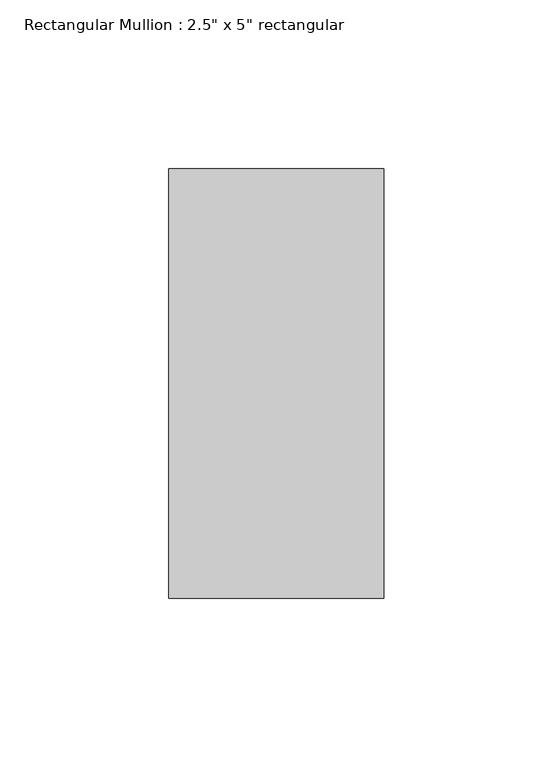
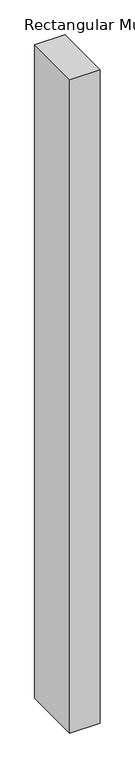
"""IFC4 building model written with IfcOpenShell, lengths in millimetres: member geometry."""

from ifc_helpers import new_model, si_unit, frame, origin, place, context, project, spatial, polyline, outline, extrude, source, transform, mapped, element, save


def member_4b9f21bc(model_context):
    return source(origin(), model_context, "Body", "SweptSolid", [
        extrude(outline(polyline([(31.75, 63.5), (31.75, -63.5), (-31.75, -63.5), (-31.75, 63.5), (31.75, 63.5)])), frame((0.0, 0.0, -1446.9422272), z_axis=(0.0, 0.0, 1.0), x_axis=(1.0, 0.0, 0.0)), (0.0, 0.0, 1.0), 1446.9422272),
    ])


if __name__ == "__main__":
    model = new_model("IFC4")
    model_context = context("Model", 3, world=origin())
    ifc_project = project(units=[si_unit("LENGTHUNIT", "METRE", prefix="MILLI")], contexts=[model_context])
    site = spatial("IfcSite", under=ifc_project)
    building = spatial("IfcBuilding", under=site)
    placement = place(None, origin())
    member_shape = member_4b9f21bc(model_context)
    element("IfcMember", 1, ObjectType="Rectangular Mullion : 2.5\" x 5\" rectangular", at=placement, inside=building, context=model_context, shape_type="MappedRepresentation", body=[
        mapped(member_shape, transform((0.0, 0.0, 0.0), x_axis=(1.0, 0.0, 0.0), y_axis=(0.0, 1.0, 0.0), z_axis=(0.0, 0.0, 1.0))),
    ])
    save(model, "model.ifc")

# Revit data of these elements
# Type "Rectangular Mullion : 2.5\" x 5\" rectangular"
#   built-in parameter 1007304 = 0.416667 (stored number, unit not read)
#   built-in parameter 1007301 = 0.104167 (stored number, unit not read)
#   built-in parameter 1007300 = 0.104167 (stored number, unit not read)
# Element 1 (IfcMember, "Rectangular Mullion : 2.5\" x 5\" rectangular")
#   Materials on its faces: "Aluminum"
# Materials
#   "Aluminum": class "Metal", colour RGB 247 247 247, transparency 0, Description = "Aluminum 6061", Cost = 0
